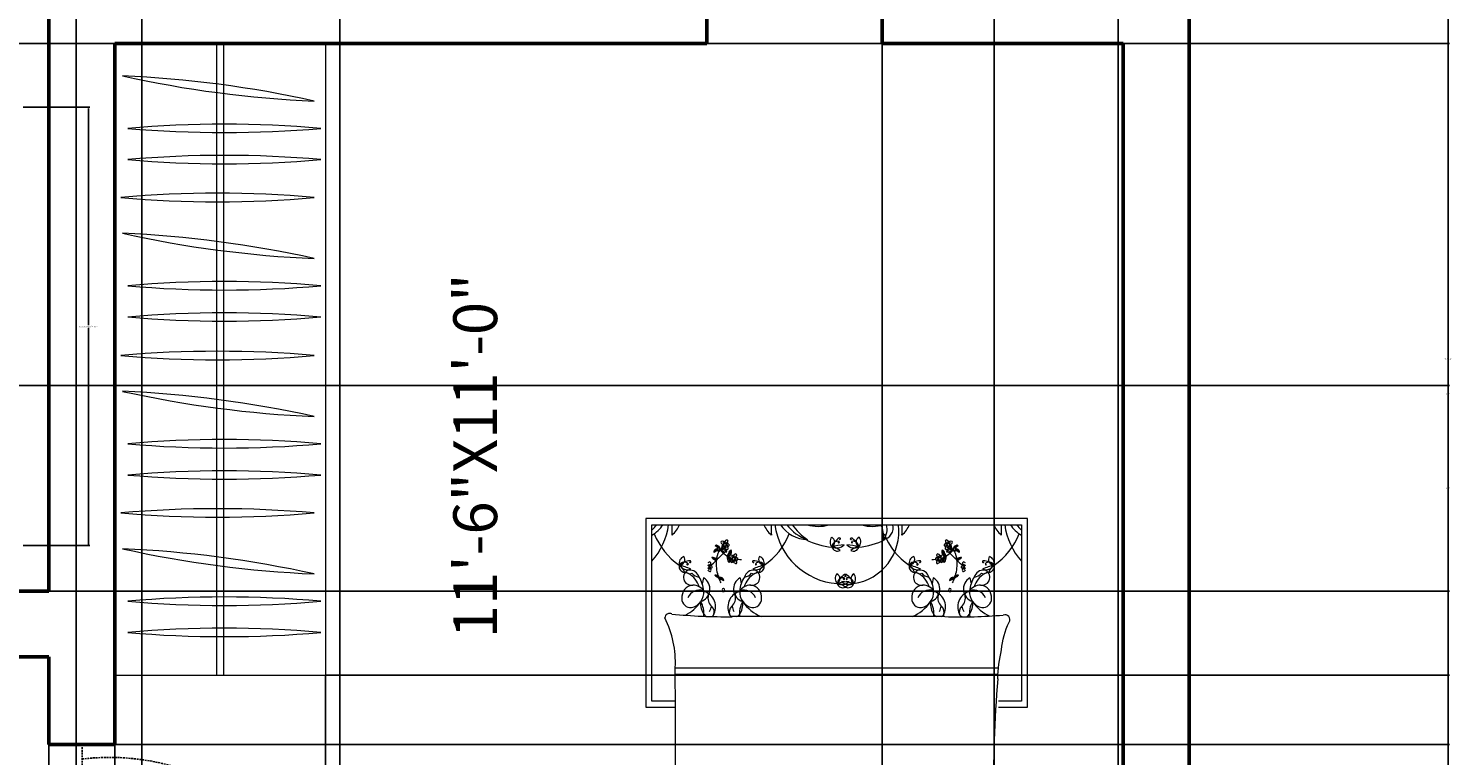
# Model space of a CAD drawing. Units: inches. Extents: x 3 to 576, y -689 to 51.
# Tile 20 of 21: x 381 to 576, y -148 to -48. Entities that reach past the tile are written whole.
import ezdxf

# ---------------------------------------------------------------- set-up
doc = ezdxf.new("R2010")
doc.units = ezdxf.units.IN
doc.header["$MEASUREMENT"] = 0
doc.linetypes.add('DASHED2', pattern=[0.375, 0.25, -0.125])
for name, color, linetype, lineweight in [('A-ANNO-DIMS', 2, 'Continuous', 18), ('A-AREA-IDEN', 7, 'Continuous', 18), ('A-DOOR', 4, 'DASHED2', 25), ('A-FURN', 8, 'Continuous', 18), ('A-WALL', 7, 'Continuous', 50)]:
    doc.layers.add(name, color=color, linetype=linetype, lineweight=lineweight)
doc.styles.get("Standard").update_dxf_attribs({"font": 'arial.ttf'})
doc.dimstyles.get("Standard").update_dxf_attribs({"dimtxt": 0.18, "dimasz": 0.18, "dimexe": 0.18, "dimexo": 0.0625, "dimgap": 0.09, "dimtad": 0, "dimtih": 1, "dimtoh": 1, "dimdec": 0, "dimzin": 0, "dimdsep": 46, "dimlunit": 3, "dimtxsty": 'Standard', "dimcen": 0.09, "dimadec": 0, "dimazin": 0, "dimtfac": 1, "dimtdec": 0, "dimtofl": 0, "dimtmove": 0, "dimatfit": 3, "dimfxl": 1, "dimtolj": 1, "dimtzin": 0, "dimarcsym": 0})

# ---------------------------------------------------------------- blocks, each defined once
blk = doc.blocks.new('DOOR-SWING-900')
for p, q in [((35.95, 36), (35.95, 34)), ((36, 2), (35.95, 34)), ((36, 2), (0, 2)), ((36, 0), (36, 2))]:
    blk.add_line(p, q)
blk.add_arc((32.22, 2), 32.22, 83.347, 180)
blk = doc.blocks.new('*D35')
at = {"layer": 'A-ANNO-DIMS', "color": 0, "lineweight": -2, "transparency": 16777216}
for p, q in [((380.75, -59.06), (389.87, -59.06)), ((389.69, -59.24), (389.69, -88.89)), ((389.69, -118.91), (389.69, -89.26)), ((380.75, -119.09), (389.87, -119.09))]:
    blk.add_line(p, q, dxfattribs=at)
at = {"layer": 'A-ANNO-DIMS', "color": 0, "transparency": 16777216}
for points in [[(389.66, -59.24), (389.72, -59.24), (389.69, -59.06)], [(389.66, -118.91), (389.72, -118.91), (389.69, -119.09)]]:
    blk.add_solid(points, dxfattribs=at)
at = {"layer": 'Defpoints', "color": 0, "transparency": 16777216}
for p in [(380.69, -59.06), (389.69, -59.06), (380.69, -119.09)]:
    blk.add_point(p, dxfattribs=at)
at = {"layer": 'A-ANNO-DIMS', "color": 0, "transparency": 16777216, "insert": (389.69, -89.08), "char_height": 0.18, "attachment_point": 5}
blk.add_mtext('\\A1;3-SEAT SOFA 5\'-0" TYP.', dxfattribs=at)
blk = doc.blocks.new('*D39')
at = {"layer": 'A-ANNO-DIMS', "color": 0, "lineweight": -2, "transparency": 16777216}
for p, q in [((540.36, 15.69), (575.92, 15.69)), ((575.74, 15.51), (575.74, -318.63)), ((575.74, -653.13), (575.74, -318.99)), ((540.36, -653.31), (575.92, -653.31))]:
    blk.add_line(p, q, dxfattribs=at)
at = {"layer": 'A-ANNO-DIMS', "color": 0, "transparency": 16777216}
for points in [[(575.71, 15.51), (575.77, 15.51), (575.74, 15.69)], [(575.71, -653.13), (575.77, -653.13), (575.74, -653.31)]]:
    blk.add_solid(points, dxfattribs=at)
at = {"layer": 'Defpoints', "color": 0, "transparency": 16777216}
for p in [(540.29, 15.69), (540.29, -653.31), (575.74, -653.31)]:
    blk.add_point(p, dxfattribs=at)
at = {"layer": 'A-ANNO-DIMS', "color": 0, "transparency": 16777216, "insert": (575.74, -318.81), "char_height": 0.18, "attachment_point": 5}
blk.add_mtext('\\A1;55\'-9"', dxfattribs=at)
blk = doc.blocks.new('*D64')
at = {"layer": 'A-ANNO-DIMS', "color": 0, "lineweight": -2, "transparency": 16777216}
for p, q in [((540.23, 15.69), (2.66, 15.69)), ((2.84, 15.51), (2.84, -17.13)), ((2.84, -50.13), (2.84, -17.49)), ((531.23, -50.31), (2.66, -50.31))]:
    blk.add_line(p, q, dxfattribs=at)
at = {"layer": 'A-ANNO-DIMS', "color": 0, "transparency": 16777216}
for points in [[(2.81, 15.51), (2.87, 15.51), (2.84, 15.69)], [(2.81, -50.13), (2.87, -50.13), (2.84, -50.31)]]:
    blk.add_solid(points, dxfattribs=at)
at = {"layer": 'Defpoints', "color": 0, "transparency": 16777216}
for p in [(540.29, 15.69), (2.84, -50.31), (531.29, -50.31)]:
    blk.add_point(p, dxfattribs=at)
at = {"layer": 'A-ANNO-DIMS', "color": 0, "transparency": 16777216, "insert": (2.84, -17.31), "char_height": 0.18, "attachment_point": 5}
blk.add_mtext('\\A1;5\'-6"', dxfattribs=at)
blk = doc.blocks.new('*D65')
at = {"layer": 'A-ANNO-DIMS', "color": 0, "lineweight": -2, "transparency": 16777216}
for p, q in [((531.23, -50.31), (2.66, -50.31)), ((2.84, -50.49), (2.84, -116.13)), ((2.84, -182.13), (2.84, -116.49)), ((531.23, -182.31), (2.66, -182.31))]:
    blk.add_line(p, q, dxfattribs=at)
at = {"layer": 'A-ANNO-DIMS', "color": 0, "transparency": 16777216}
for points in [[(2.81, -50.49), (2.87, -50.49), (2.84, -50.31)], [(2.81, -182.13), (2.87, -182.13), (2.84, -182.31)]]:
    blk.add_solid(points, dxfattribs=at)
at = {"layer": 'Defpoints', "color": 0, "transparency": 16777216}
for p in [(531.29, -50.31), (2.84, -182.31), (531.29, -182.31)]:
    blk.add_point(p, dxfattribs=at)
at = {"layer": 'A-ANNO-DIMS', "color": 0, "transparency": 16777216, "insert": (2.84, -116.31), "char_height": 0.18, "attachment_point": 5}
blk.add_mtext('\\A1;11\'-0"', dxfattribs=at)
blk = doc.blocks.new('*D87')
at = {"layer": 'A-ANNO-DIMS', "color": 0, "lineweight": -2, "transparency": 16777216}
for p, q in [((195.85, -97.15), (575.92, -97.15)), ((575.74, -97.33), (575.74, -111.05)), ((575.74, -125.13), (575.74, -111.41)), ((195.85, -125.31), (575.92, -125.31))]:
    blk.add_line(p, q, dxfattribs=at)
at = {"layer": 'A-ANNO-DIMS', "color": 0, "transparency": 16777216}
for points in [[(575.71, -97.33), (575.77, -97.33), (575.74, -97.15)], [(575.71, -125.13), (575.77, -125.13), (575.74, -125.31)]]:
    blk.add_solid(points, dxfattribs=at)
at = {"layer": 'Defpoints', "color": 0, "transparency": 16777216}
for p in [(195.78, -97.15), (575.74, -97.15), (195.78, -125.31)]:
    blk.add_point(p, dxfattribs=at)
at = {"layer": 'A-ANNO-DIMS', "color": 0, "transparency": 16777216, "insert": (575.74, -111.23), "char_height": 0.18, "attachment_point": 5}
blk.add_mtext('\\A1;2\'-4"', dxfattribs=at)
blk = doc.blocks.new('*D94')
at = {"layer": 'A-ANNO-DIMS', "color": 0, "lineweight": -2, "transparency": 16777216}
for p, q in [((393.29, -136.9), (393.29, -688.94)), ((422.14, -136.9), (422.14, -688.94)), ((393.47, -688.76), (407.39, -688.76)), ((421.96, -688.76), (408.05, -688.76))]:
    blk.add_line(p, q, dxfattribs=at)
at = {"layer": 'A-ANNO-DIMS', "color": 0, "transparency": 16777216}
for points in [[(393.47, -688.73), (393.47, -688.79), (393.29, -688.76)], [(421.96, -688.73), (421.96, -688.79), (422.14, -688.76)]]:
    blk.add_solid(points, dxfattribs=at)
at = {"layer": 'Defpoints', "color": 0, "transparency": 16777216}
for p in [(393.29, -136.84), (422.14, -136.84), (422.14, -688.76)]:
    blk.add_point(p, dxfattribs=at)
at = {"layer": 'A-ANNO-DIMS', "color": 0, "transparency": 16777216, "insert": (407.72, -688.76), "char_height": 0.18, "attachment_point": 5}
blk.add_mtext('\\A1;2\'-5"', dxfattribs=at)
blk = doc.blocks.new('*D95')
at = {"layer": 'A-ANNO-DIMS', "color": 0, "lineweight": -2, "transparency": 16777216}
for p, q in [((422.2, -50.31), (575.92, -50.31)), ((575.74, -50.49), (575.74, -93.39)), ((575.74, -136.66), (575.74, -93.76)), ((422.2, -136.84), (575.92, -136.84))]:
    blk.add_line(p, q, dxfattribs=at)
at = {"layer": 'A-ANNO-DIMS', "color": 0, "transparency": 16777216}
for points in [[(575.71, -50.49), (575.77, -50.49), (575.74, -50.31)], [(575.71, -136.66), (575.77, -136.66), (575.74, -136.84)]]:
    blk.add_solid(points, dxfattribs=at)
at = {"layer": 'Defpoints', "color": 0, "transparency": 16777216}
for p in [(422.14, -50.31), (422.14, -136.84), (575.74, -136.84)]:
    blk.add_point(p, dxfattribs=at)
at = {"layer": 'A-ANNO-DIMS', "color": 0, "transparency": 16777216, "insert": (575.74, -93.58), "char_height": 0.18, "attachment_point": 5}
blk.add_mtext('\\A1;7\'-2 1/2"', dxfattribs=at)
blk = doc.blocks.new('*D96')
at = {"layer": 'A-ANNO-DIMS', "color": 0, "lineweight": -2, "transparency": 16777216}
for p, q in [((397.02, -506.04), (397.02, 51.32)), ((397.2, 51.14), (410.22, 51.14)), ((423.91, 51.14), (410.89, 51.14)), ((424.09, -506.04), (424.09, 51.32))]:
    blk.add_line(p, q, dxfattribs=at)
at = {"layer": 'A-ANNO-DIMS', "color": 0, "transparency": 16777216}
for points in [[(397.2, 51.17), (397.2, 51.11), (397.02, 51.14)], [(423.91, 51.17), (423.91, 51.11), (424.09, 51.14)]]:
    blk.add_solid(points, dxfattribs=at)
at = {"layer": 'Defpoints', "color": 0, "transparency": 16777216}
for p in [(424.09, 51.14), (397.02, -506.1), (424.09, -506.1)]:
    blk.add_point(p, dxfattribs=at)
at = {"layer": 'A-ANNO-DIMS', "color": 0, "transparency": 16777216, "insert": (410.56, 51.14), "char_height": 0.18, "attachment_point": 5}
blk.add_mtext('\\A1;2\'-3"', dxfattribs=at)
blk = doc.blocks.new('*D103')
at = {"layer": 'A-ANNO-DIMS', "color": 0, "lineweight": -2, "transparency": 16777216}
for p, q in [((498.29, -50.37), (498.29, -688.94)), ((531.29, -50.37), (531.29, -688.94)), ((498.47, -688.76), (514.46, -688.76)), ((531.11, -688.76), (515.12, -688.76))]:
    blk.add_line(p, q, dxfattribs=at)
at = {"layer": 'A-ANNO-DIMS', "color": 0, "transparency": 16777216}
for points in [[(498.47, -688.73), (498.47, -688.79), (498.29, -688.76)], [(531.11, -688.73), (531.11, -688.79), (531.29, -688.76)]]:
    blk.add_solid(points, dxfattribs=at)
at = {"layer": 'Defpoints', "color": 0, "transparency": 16777216}
for p in [(498.29, -50.31), (531.29, -50.31), (531.29, -688.76)]:
    blk.add_point(p, dxfattribs=at)
at = {"layer": 'A-ANNO-DIMS', "color": 0, "transparency": 16777216, "insert": (514.79, -688.76), "char_height": 0.18, "attachment_point": 5}
blk.add_mtext('\\A1;2\'-9"', dxfattribs=at)
blk = doc.blocks.new('*D104')
at = {"layer": 'A-ANNO-DIMS', "color": 0, "lineweight": -2, "transparency": 16777216}
for p, q in [((393.36, -50.31), (575.92, -50.31)), ((575.74, -50.49), (575.74, -98.13)), ((575.74, -146.13), (575.74, -98.49)), ((393.36, -146.31), (575.92, -146.31))]:
    blk.add_line(p, q, dxfattribs=at)
at = {"layer": 'A-ANNO-DIMS', "color": 0, "transparency": 16777216}
for points in [[(575.71, -50.49), (575.77, -50.49), (575.74, -50.31)], [(575.71, -146.13), (575.77, -146.13), (575.74, -146.31)]]:
    blk.add_solid(points, dxfattribs=at)
at = {"layer": 'Defpoints', "color": 0, "transparency": 16777216}
for p in [(393.29, -50.31), (393.29, -146.31), (575.74, -146.31)]:
    blk.add_point(p, dxfattribs=at)
at = {"layer": 'A-ANNO-DIMS', "color": 0, "transparency": 16777216, "insert": (575.74, -98.31), "char_height": 0.18, "attachment_point": 5}
blk.add_mtext('\\A1;8\'-0"', dxfattribs=at)
blk = doc.blocks.new('*D116')
at = {"layer": 'A-ANNO-DIMS', "color": 0, "lineweight": -2, "transparency": 16777216}
for p, q in [((360.29, -134.37), (360.29, -688.94)), ((384.29, -134.37), (384.29, -688.94)), ((360.47, -688.76), (371.96, -688.76)), ((384.11, -688.76), (372.62, -688.76))]:
    blk.add_line(p, q, dxfattribs=at)
at = {"layer": 'A-ANNO-DIMS', "color": 0, "transparency": 16777216}
for points in [[(360.47, -688.73), (360.47, -688.79), (360.29, -688.76)], [(384.11, -688.73), (384.11, -688.79), (384.29, -688.76)]]:
    blk.add_solid(points, dxfattribs=at)
at = {"layer": 'Defpoints', "color": 0, "transparency": 16777216}
for p in [(360.29, -134.31), (384.29, -134.31), (384.29, -688.76)]:
    blk.add_point(p, dxfattribs=at)
at = {"layer": 'A-ANNO-DIMS', "color": 0, "transparency": 16777216, "insert": (372.29, -688.76), "char_height": 0.18, "attachment_point": 5}
blk.add_mtext('\\A1;2\'-0"', dxfattribs=at)
blk = doc.blocks.new('*D118')
at = {"layer": 'A-ANNO-DIMS', "color": 0, "lineweight": -2, "transparency": 16777216}
for p, q in [((352.02, -506.25), (352.02, 51.32)), ((352.2, 51.14), (369.69, 51.14)), ((387.84, 51.14), (370.35, 51.14)), ((388.02, -506.25), (388.02, 51.32))]:
    blk.add_line(p, q, dxfattribs=at)
at = {"layer": 'A-ANNO-DIMS', "color": 0, "transparency": 16777216}
for points in [[(352.2, 51.17), (352.2, 51.11), (352.02, 51.14)], [(387.84, 51.17), (387.84, 51.11), (388.02, 51.14)]]:
    blk.add_solid(points, dxfattribs=at)
at = {"layer": 'Defpoints', "color": 0, "transparency": 16777216}
for p in [(388.02, 51.14), (352.02, -506.31), (388.02, -506.31)]:
    blk.add_point(p, dxfattribs=at)
at = {"layer": 'A-ANNO-DIMS', "color": 0, "transparency": 16777216, "insert": (370.02, 51.14), "char_height": 0.18, "attachment_point": 5}
blk.add_mtext('\\A1;3\'-0"', dxfattribs=at)
blk = doc.blocks.new('*D124')
at = {"layer": 'A-ANNO-DIMS', "color": 0, "lineweight": -2, "transparency": 16777216}
for p, q in [((513.61, -235.44), (513.61, 51.32)), ((513.79, 51.14), (521.77, 51.14)), ((530.39, 51.14), (522.41, 51.14)), ((530.57, -227.22), (530.57, 51.32))]:
    blk.add_line(p, q, dxfattribs=at)
at = {"layer": 'A-ANNO-DIMS', "color": 0, "transparency": 16777216}
for points in [[(513.79, 51.17), (513.79, 51.11), (513.61, 51.14)], [(530.39, 51.17), (530.39, 51.11), (530.57, 51.14)]]:
    blk.add_solid(points, dxfattribs=at)
at = {"layer": 'Defpoints', "color": 0, "transparency": 16777216}
for p in [(530.57, 51.14), (530.57, -227.28), (513.61, -235.5)]:
    blk.add_point(p, dxfattribs=at)
at = {"layer": 'A-ANNO-DIMS', "color": 0, "transparency": 16777216, "insert": (522.09, 51.14), "char_height": 0.18, "attachment_point": 5}
blk.add_mtext('\\A1;1\'-5"', dxfattribs=at)

msp = doc.modelspace()

# ---------------------------------------------------------------- linework, layer by layer
at = {"layer": 'A-FURN'}
for p, q in [((393.29, -50.31), (393.29, -136.84)), ((393.29, -50.31), (422.14, -50.31)), ((407.24, -50.31), (407.24, -136.84)), ((408.2, -50.31), (408.2, -136.84)), ((422.14, -50.31), (422.14, -136.84)), ((465.95, -115.39), (465.95, -141.21)), ((518.2, -115.39), (465.95, -115.39)), ((466.78, -116.22), (517.37, -116.22)), ((466.78, -140.38), (466.78, -116.22)), ((517.37, -116.22), (517.37, -140.38)), ((518.2, -141.21), (518.2, -115.39)), ((473.84, -123.49), (473.69, -124.3)), ((478.85, -123.49), (479.01, -124.3)), ((505.3, -123.49), (505.14, -124.3)), ((510.31, -123.49), (510.47, -124.3)), ((506.87, -128.81), (477.78, -128.81)), ((514.22, -135.85), (470, -135.85)), ((393.29, -136.84), (422.14, -136.84)), ((514.15, -136.74), (470, -136.74)), ((465.95, -141.21), (470.01, -141.21)), ((470, -140.38), (466.78, -140.38)), ((517.37, -140.38), (514.21, -140.38)), ((514.23, -141.21), (518.2, -141.21))]:
    msp.add_line(p, q, dxfattribs=at)
for points in [[(470.03, -149.36, -0.001242), (470, -135.76, 0.127202), (468.56, -128.99)], [(514.13, -137.31, -0.056112), (514.65, -133.36, -0.095341), (515.66, -129.56)]]:
    msp.add_lwpolyline(points, format="xyb", dxfattribs=at)
for centre in [(476.79, -118.97), (477.98, -120.89), (506.17, -120.89), (507.36, -118.97)]:
    msp.add_circle(centre, 0.183, dxfattribs=at)
for centre, radius, start, end in [((427.2, 93.42), 151.77, 257.508, 267.5023), ((387.76, -206.38), 151.77, 77.508, 87.5023), ((408.29, -213.14), 151.77, 85.0028, 94.9972), ((408.29, 89.25), 151.77, 265.0028, 274.9972), ((408.29, -217.41), 151.77, 85.0028, 94.9972), ((408.29, 84.98), 151.77, 265.0028, 274.9972), ((407.36, -222.6), 151.77, 85.0028, 94.9972), ((407.36, 79.78), 151.77, 265.0028, 274.9972), ((427.2, 71.86), 151.77, 257.508, 267.5023), ((387.76, -227.94), 151.77, 77.508, 87.5023), ((408.29, -234.69), 151.77, 85.0028, 94.9972), ((408.29, 67.69), 151.77, 265.0028, 274.9972), ((408.29, -238.97), 151.77, 85.0028, 94.9972), ((408.29, 63.42), 151.77, 265.0028, 274.9972), ((407.36, -244.24), 151.77, 85.0028, 94.9972), ((407.36, 58.14), 151.77, 265.0028, 274.9972), ((387.76, -249.58), 151.77, 77.508, 87.5023), ((427.2, 50.22), 151.77, 257.508, 267.5023), ((408.29, -256.33), 151.77, 85.0028, 94.9972), ((408.29, 46.05), 151.77, 265.0028, 274.9972), ((408.29, -260.61), 151.77, 85.0028, 94.9972), ((408.29, 41.78), 151.77, 265.0028, 274.9972), ((407.36, -265.8), 151.77, 85.0028, 94.9972), ((407.36, 36.58), 151.77, 265.0028, 274.9972), ((462.87, -112.86), 5.68, 313.5186, 323.6964), ((464.51, -113.71), 4.56, 299.8884, 326.5383), ((459.81, -114.96), 9.36, 318.1144, 352.255), ((467.06, -114.76), 3.81, 311.0454, 337.4453), ((456.64, -116.81), 12.95, 356.3481, 2.5919), ((485.63, -114.76), 3.81, 202.5547, 228.9546), ((496.06, -116.81), 12.95, 177.4081, 183.6519), ((492.88, -114.96), 9.36, 187.745, 265.5377), ((488.19, -113.71), 4.56, 213.4617, 268.728), ((489.83, -112.86), 5.68, 216.3036, 252.1496), ((492.82, -111.26), 8.45, 215.947, 235.9877), ((489.55, -111.3), 5.15, 252.9798, 286.4569), ((491.59, -108.65), 7.61, 264.3643, 265.6213), ((495.6, -103.44), 13.6, 250.0972, 250.2783), ((493.35, -117.12), 7.24, 278.1803, 7.1364), ((496.99, -111.3), 5.15, 253.5431, 287.0202), ((494.95, -108.65), 7.61, 274.3787, 275.6357), ((490.94, -103.44), 13.6, 289.7217, 289.9028), ((494.29, -117.79), 4.19, 353.3805, 21.883), ((498.13, -116.62), 1.68, 280.9261, 13.6102), ((496.87, -116.85), 2.12, 318.0951, 17.1391), ((488.09, -116.81), 12.95, 356.3481, 2.5919), ((498.52, -114.76), 3.81, 311.0454, 337.4453), ((517.09, -114.76), 3.81, 202.5547, 228.9546), ((527.51, -116.81), 12.95, 177.4081, 183.6519), ((524.34, -114.96), 9.36, 187.745, 221.8856), ((519.64, -113.71), 4.56, 213.4617, 240.1116), ((521.28, -112.86), 5.68, 216.3036, 226.4814), ((475.83, -114.04), 9.36, 201.4092, 235.6135), ((476.41, -118.63), 0.181, 134.3732, 211.9501), ((476.74, -118.42), 0.575, 211.9501, 255.2442), ((476.42, -118.83), 0.36, 8.5614, 112.5914), ((476.52, -118.82), 0.121, 352.868, 97.094), ((477.04, -118.63), 0.301, 100.9597, 208.7804), ((477.36, -119.03), 0.554, 132.3896, 156.5724), ((476.78, -118.47), 0.424, 291.6382, 4.947), ((477.07, -118.45), 0.14, 4.947, 127.5263), ((476.87, -114.04), 9.36, 304.3865, 338.5908), ((492.17, -109.95), 9.36, 242.5854, 265.5377), ((492.21, -118.58), 1.04, 140.8855, 222.2127), ((491.03, -118.62), 0.782, 301.6373, 61.4609), ((493.68, -120.05), 2.37, 121.989, 161.0841), ((492.2, -119.25), 0.766, 76.148, 182.2415), ((492.36, -118.61), 0.101, 140.0755, 76.148), ((492.48, -118.14), 0.116, 288.4408, 121.989), ((492.5, -118.2), 0.0565, 171.9833, 288.4408), ((494.06, -118.14), 0.116, 58.011, 251.5592), ((494.04, -118.2), 0.0565, 251.5592, 8.0167), ((494.17, -118.64), 0.061, 103.9791, 39.8091), ((492.86, -120.05), 2.37, 18.9159, 58.011), ((494.34, -119.25), 0.766, 357.7585, 103.852), ((495.51, -118.62), 0.782, 118.5391, 238.3627), ((494.33, -118.58), 1.04, 317.7873, 39.1145), ((494.37, -109.95), 9.36, 274.4623, 297.4146), ((507.28, -114.04), 9.36, 201.4092, 235.6135), ((507.08, -118.45), 0.14, 52.4737, 175.053), ((507.37, -118.47), 0.424, 175.053, 248.3618), ((506.79, -119.03), 0.554, 23.4276, 47.6104), ((507.11, -118.63), 0.301, 331.2196, 79.0403), ((507.73, -118.83), 0.36, 67.4086, 171.4386), ((507.63, -118.82), 0.121, 82.906, 187.132), ((507.41, -118.42), 0.575, 284.7558, 328.0499), ((507.74, -118.63), 0.181, 328.0499, 45.6268), ((508.33, -114.04), 9.36, 304.3865, 338.5908), ((387.76, -271.14), 151.77, 77.508, 87.5023), ((427.2, 28.66), 151.77, 257.508, 267.5023), ((471.55, -121.54), 1.04, 110.9613, 192.2885), ((470.52, -120.98), 0.782, 271.7131, 31.5367), ((475.46, -119.9), 0.204, 123.0979, 213.1364), ((475.81, -120.2), 0.552, 92.3172, 160.5201), ((478.34, -124.39), 5.33, 121.1156, 124.8118), ((475.75, -119.99), 0.475, 82.6008, 147.1845), ((475.61, -119.24), 0.204, 55.6077, 145.6462), ((475.47, -119.67), 0.552, 21.7087, 93.0299), ((472.57, -123.61), 5.33, 53.6254, 57.3216), ((475.69, -120.01), 0.211, 45.7354, 121.1156), ((478.56, -121.35), 2.98, 150.7959, 175.244), ((482.85, -127.69), 9.79, 127.8256, 137.7588), ((475.64, -119.53), 0.475, 342.8042, 79.6943), ((475.6, -119.49), 0.211, 338.2452, 53.6254), ((475.95, -119.62), 0.159, 158.2452, 340.6395), ((475.95, -119.74), 0.159, 225.7354, 48.1297), ((478.94, -118.29), 3.18, 201.7087, 206.2181), ((476.41, -120.46), 0.832, 40.9365, 112.7695), ((476.14, -120.18), 0.49, 49.3812, 95.5456), ((478.56, -121.35), 2.98, 137.5083, 145.9967), ((476.49, -119.99), 0.506, 61.1838, 141.6792), ((478.87, -117.4), 3.57, 220.182, 239.456), ((476.59, -119.22), 0.249, 88.5719, 233.8954), ((476.56, -119.29), 0.179, 228.2946, 6.2474), ((476.84, -119.37), 0.589, 229.3812, 289.9959), ((476.39, -119.08), 0.251, 298.8493, 359.9355), ((476.45, -119.29), 0.287, 4.2123, 48.1587), ((477.04, -119.25), 0.304, 183.635, 258.4363), ((476.46, -120.08), 0.604, 15.6484, 62.2957), ((477, -119.14), 0.174, 178.1325, 268.8919), ((477.12, -119.1), 0.299, 42.3208, 130.2111), ((477.19, -118.79), 0.377, 226.3462, 279.6513), ((476.8, -119.49), 0.439, 7.4968, 71.2737), ((477.12, -118.4), 0.597, 254.2829, 276.9148), ((477.1, -119.47), 0.141, 215.0752, 14.7644), ((476.8, -119.69), 0.832, 287.889, 359.722), ((476.78, -120.08), 0.49, 305.1128, 351.2773), ((477.03, -120.98), 0.506, 3.8774, 87.1501), ((476.67, -120.78), 0.49, 352.0748, 38.2393), ((476.59, -121.16), 0.832, 343.6301, 55.4631), ((477.18, -119.99), 0.506, 271.4625, 339.4747), ((477.23, -119.01), 0.157, 279.6513, 42.3208), ((477.84, -120.24), 0.589, 110.6625, 171.2773), ((477.6, -120.55), 0.181, 134.3732, 211.9501), ((478.87, -117.4), 3.57, 246.1523, 246.9499), ((477.94, -120.34), 0.575, 211.9501, 255.2442), ((477.61, -120.75), 0.36, 8.5614, 112.5914), ((477.09, -119.95), 0.604, 338.3627, 25.0101), ((477.71, -120.74), 0.121, 352.868, 97.094), ((478.23, -120.56), 0.301, 100.9597, 208.7804), ((478.56, -120.96), 0.554, 132.3896, 156.5724), ((477.98, -120.4), 0.424, 291.6382, 4.947), ((478.26, -120.37), 0.14, 4.947, 127.5263), ((482.18, -120.98), 0.782, 148.4633, 268.2869), ((481.14, -121.54), 1.04, 347.7115, 69.0387), ((493.4, -125.53), 6.55, 92.7418, 107.407), ((492.05, -117.93), 1.48, 245.6899, 314.4589), ((491.4, -120.88), 1.6, 44.6273, 88.5415), ((492.18, -119.06), 0.776, 196.1963, 296.9726), ((493.14, -125.53), 6.55, 72.593, 87.2582), ((494.49, -117.93), 1.48, 225.5411, 294.3101), ((495.14, -120.88), 1.6, 91.4585, 135.3727), ((494.36, -119.06), 0.776, 243.0274, 343.8037), ((503.01, -121.54), 1.04, 110.9613, 192.2885), ((501.97, -120.98), 0.782, 271.7131, 31.5367), ((505.89, -120.37), 0.14, 52.4737, 175.053), ((506.17, -120.4), 0.424, 175.053, 248.3618), ((505.59, -120.96), 0.554, 23.4276, 47.6104), ((505.92, -120.56), 0.301, 331.2196, 79.0403), ((506.54, -120.75), 0.36, 67.4086, 171.4386), ((506.44, -120.74), 0.121, 82.906, 187.132), ((506.22, -120.34), 0.575, 284.7558, 328.0499), ((507.06, -119.95), 0.604, 154.9899, 201.6373), ((506.98, -119.99), 0.506, 200.5253, 268.5375), ((507.35, -119.69), 0.832, 180.278, 252.111), ((506.31, -120.24), 0.589, 8.7227, 69.3375), ((507.12, -120.98), 0.506, 92.8499, 176.1226), ((506.55, -120.55), 0.181, 328.0499, 45.6268), ((505.28, -117.4), 3.57, 293.0501, 293.8477), ((507.56, -121.16), 0.832, 124.5369, 196.3699), ((506.93, -119.01), 0.157, 137.6792, 260.3487), ((507.03, -119.1), 0.299, 49.7889, 137.6792), ((507.37, -120.08), 0.49, 188.7227, 234.8872), ((506.96, -118.79), 0.377, 260.3487, 313.6538), ((507.05, -119.47), 0.141, 165.2356, 324.9248), ((507.35, -119.49), 0.439, 108.7263, 172.5032), ((507.03, -118.4), 0.597, 263.0852, 285.7171), ((507.48, -120.78), 0.49, 141.7607, 187.9252), ((505.28, -117.4), 3.57, 300.544, 319.818), ((507.69, -120.08), 0.604, 117.7043, 164.3516), ((507.74, -120.46), 0.832, 67.2305, 139.0635), ((507.31, -119.37), 0.589, 250.0041, 310.6188), ((507.15, -119.14), 0.174, 271.1081, 1.8675), ((507.11, -119.25), 0.304, 281.5637, 356.365), ((501.3, -127.69), 9.79, 42.2412, 52.1744), ((507.7, -119.29), 0.287, 131.8413, 175.7877), ((507.59, -119.29), 0.179, 173.7526, 311.7054), ((507.66, -119.99), 0.506, 38.3208, 118.8162), ((507.76, -119.08), 0.251, 180.0645, 241.1507), ((507.56, -119.22), 0.249, 306.1046, 91.4281), ((508.01, -120.18), 0.49, 84.4544, 130.6188), ((505.59, -121.35), 2.98, 34.0033, 42.4917), ((508.51, -119.53), 0.475, 100.3057, 197.1958), ((508.2, -119.74), 0.159, 131.8703, 314.2646), ((508.2, -119.62), 0.159, 199.3605, 21.7548), ((505.21, -118.29), 3.18, 333.7819, 338.2913), ((508.68, -119.67), 0.552, 86.9701, 158.2913), ((505.59, -121.35), 2.98, 4.756, 29.2041), ((508.46, -120.01), 0.211, 58.8844, 134.2646), ((508.55, -119.49), 0.211, 126.3746, 201.7548), ((508.4, -119.99), 0.475, 32.8155, 97.3992), ((508.34, -120.2), 0.552, 19.4799, 87.6828), ((508.54, -119.24), 0.204, 34.3538, 124.3923), ((511.58, -123.61), 5.33, 122.6784, 126.3746), ((505.81, -124.39), 5.33, 55.1882, 58.8844), ((508.69, -119.9), 0.204, 326.8636, 56.9021), ((513.63, -120.98), 0.782, 148.4633, 268.2869), ((512.6, -121.54), 1.04, 347.7115, 69.0387), ((471.29, -121.95), 0.776, 166.272, 267.0484), ((472.1, -123.54), 2.37, 92.0648, 131.1598), ((471.22, -122.12), 0.766, 46.2238, 152.3173), ((469.12, -128.15), 6.55, 62.8176, 77.4827), ((471.74, -120.9), 1.48, 215.7657, 284.5347), ((469.71, -123.13), 1.6, 14.7031, 58.6173), ((472.2, -123.43), 1.08, 109.1312, 279.736), ((471.98, -122.27), 0.659, 216.7319, 296.0245), ((471.68, -121.64), 0.101, 110.2817, 46.2238), ((471.95, -123.76), 1.34, 15.6955, 94.031), ((472, -121.35), 0.0565, 142.0591, 258.5166), ((472.02, -121.29), 0.116, 258.5166, 92.0648), ((474.7, -121.64), 0.301, 100.9597, 142.2379), ((474.45, -121.98), 0.183, 273.2768, 86.7232), ((474.7, -122.26), 0.304, 217.3642, 258.4363), ((474.66, -122.15), 0.174, 178.1325, 268.8919), ((475.02, -122.04), 0.554, 132.3896, 156.5724), ((474.78, -122.11), 0.299, 42.3208, 130.2111), ((474.84, -121.8), 0.377, 226.3462, 279.6513), ((474.44, -121.48), 0.424, 291.6382, 4.947), ((474.45, -122.5), 0.439, 7.4968, 71.2737), ((474.77, -121.41), 0.597, 254.2829, 276.9148), ((474.72, -121.46), 0.14, 4.947, 127.5263), ((474.75, -122.48), 0.141, 215.0752, 14.7644), ((470.64, -116.45), 6.8, 307.9541, 316.8459), ((474.88, -122.02), 0.157, 279.6513, 42.3208), ((475.06, -122.74), 2.02, 82.8698, 91.6736), ((475.34, -120.56), 0.376, 205.5379, 258.6744), ((474.79, -121.84), 1.13, 59.344, 79.7412), ((474.55, -121.84), 1.15, 43.6929, 51.7899), ((475.26, -121.08), 0.344, 355.7131, 81.6568), ((475.07, -121.38), 0.601, 27.3659, 59.344), ((475.52, -120.98), 0.146, 202.5583, 304.2343), ((481.52, -121.5), 5.94, 176.1723, 196.4158), ((477.74, -120.93), 0.589, 172.0748, 232.6895), ((476.93, -121), 0.604, 318.342, 4.9894), ((477.78, -121.15), 0.249, 88.5719, 233.8954), ((477.76, -121.21), 0.179, 228.2946, 6.2474), ((477.59, -121), 0.251, 298.8493, 359.9355), ((477.65, -121.22), 0.287, 4.2123, 48.1587), ((478.24, -121.18), 0.304, 183.635, 258.4363), ((478.2, -121.07), 0.174, 178.1325, 268.8919), ((478.31, -121.03), 0.299, 42.3208, 130.2111), ((478.38, -120.72), 0.377, 226.3462, 279.6513), ((477.99, -121.41), 0.439, 7.4968, 71.2737), ((478.31, -120.32), 0.597, 254.2829, 276.9148), ((478.29, -121.39), 0.141, 215.0752, 14.7644), ((478.42, -120.93), 0.157, 279.6513, 42.3208), ((478.87, -117.4), 3.57, 265.2415, 272.8929), ((480.75, -123.76), 1.34, 85.969, 164.3045), ((480.49, -123.43), 1.08, 260.264, 70.8688), ((480.71, -122.27), 0.659, 243.9755, 323.2681), ((480.68, -121.29), 0.116, 87.9352, 281.4834), ((480.96, -120.9), 1.48, 255.4653, 324.2343), ((483.58, -128.15), 6.55, 102.5173, 117.1824), ((480.6, -123.54), 2.37, 48.8402, 87.9352), ((480.69, -121.35), 0.0565, 281.4834, 37.9409), ((481.48, -122.12), 0.766, 27.6827, 133.7762), ((481.03, -121.68), 0.061, 133.7729, 69.7333), ((481.4, -121.95), 0.776, 272.9516, 13.728), ((482.99, -123.13), 1.6, 121.3827, 165.2969), ((502.75, -121.95), 0.776, 166.272, 267.0484), ((503.55, -123.54), 2.37, 92.0648, 131.1598), ((502.67, -122.12), 0.766, 46.2238, 152.3173), ((501.16, -123.13), 1.6, 14.7031, 58.6173), ((503.19, -120.9), 1.48, 215.7657, 284.5347), ((500.58, -128.15), 6.55, 62.8176, 77.4827), ((503.66, -123.43), 1.08, 109.1312, 279.736), ((503.44, -122.27), 0.659, 216.7319, 296.0245), ((503.13, -121.64), 0.101, 110.2817, 46.2238), ((503.4, -123.76), 1.34, 15.6955, 94.031), ((503.46, -121.35), 0.0565, 142.0591, 258.5166), ((503.47, -121.29), 0.116, 258.5166, 92.0648), ((505.28, -117.4), 3.57, 267.1071, 274.7585), ((505.73, -120.93), 0.157, 137.6792, 260.3487), ((505.84, -121.03), 0.299, 49.7889, 137.6792), ((505.77, -120.72), 0.377, 260.3487, 313.6538), ((506.16, -121.41), 0.439, 108.7263, 172.5032), ((505.86, -121.39), 0.141, 165.2356, 324.9248), ((505.84, -120.32), 0.597, 263.0852, 285.7171), ((505.95, -121.07), 0.174, 271.1081, 1.8675), ((505.91, -121.18), 0.304, 281.5637, 356.365), ((506.5, -121.22), 0.287, 131.8413, 175.7877), ((506.4, -121.21), 0.179, 173.7526, 311.7054), ((506.56, -121), 0.251, 180.0645, 241.1507), ((506.37, -121.15), 0.249, 306.1046, 91.4281), ((507.22, -121), 0.604, 175.0106, 221.658), ((506.41, -120.93), 0.589, 307.3105, 7.9252), ((502.63, -121.5), 5.94, 343.5842, 3.8277), ((508.89, -121.08), 0.344, 98.3432, 184.2869), ((509.09, -121.38), 0.601, 120.656, 152.6341), ((508.63, -120.98), 0.146, 235.7657, 337.4417), ((513.52, -116.45), 6.8, 223.1541, 232.0459), ((509.6, -121.84), 1.15, 128.2101, 136.3071), ((509.36, -121.84), 1.13, 100.2588, 120.656), ((509.1, -122.74), 2.02, 88.3264, 97.1302), ((508.82, -120.56), 0.376, 281.3256, 334.4621), ((509.27, -122.02), 0.157, 137.6792, 260.3487), ((509.37, -122.11), 0.299, 49.7889, 137.6792), ((509.31, -121.8), 0.377, 260.3487, 313.6538), ((509.7, -122.5), 0.439, 108.7263, 172.5032), ((509.4, -122.48), 0.141, 165.2356, 324.9248), ((509.43, -121.46), 0.14, 52.4737, 175.053), ((509.71, -121.48), 0.424, 175.053, 248.3618), ((509.38, -121.41), 0.597, 263.0852, 285.7171), ((509.13, -122.04), 0.554, 23.4276, 47.6104), ((509.49, -122.15), 0.174, 271.1081, 1.8675), ((509.46, -121.64), 0.301, 37.7621, 79.0403), ((509.45, -122.26), 0.304, 281.5637, 322.6358), ((509.7, -121.98), 0.183, 93.2768, 266.7232), ((512.2, -123.76), 1.34, 85.969, 164.3045), ((511.95, -123.43), 1.08, 260.264, 70.8688), ((512.17, -122.27), 0.659, 243.9755, 323.2681), ((512.13, -121.29), 0.116, 87.9352, 281.4834), ((515.03, -128.15), 6.55, 102.5173, 117.1824), ((512.41, -120.9), 1.48, 255.4653, 324.2343), ((512.05, -123.54), 2.37, 48.8402, 87.9352), ((512.15, -121.35), 0.0565, 281.4834, 37.9409), ((512.93, -122.12), 0.766, 27.6827, 133.7762), ((512.48, -121.68), 0.061, 133.7729, 69.7333), ((514.44, -123.13), 1.6, 121.3827, 165.2969), ((512.86, -121.95), 0.776, 272.9516, 13.728), ((472.6, -126.19), 1.71, 97.1143, 185.0551), ((470.07, -125.8), 3.38, 18.2955, 58.7386), ((473.39, -121.97), 1.43, 218.4175, 263.8338), ((472.3, -126.57), 2.08, 35.9599, 87.6409), ((470.04, -125.53), 3.85, 3.4924, 33.7117), ((472.96, -125.03), 1.78, 286.8663, 60.0915), ((475.48, -125.16), 2.02, 82.8698, 91.6736), ((475.76, -122.97), 0.376, 205.5379, 258.6744), ((475.22, -124.25), 1.13, 59.344, 79.7412), ((474.98, -124.25), 1.15, 43.6929, 51.7899), ((475.68, -123.49), 0.344, 355.7131, 81.6568), ((475.49, -123.79), 0.601, 27.3659, 59.344), ((475.94, -123.4), 0.146, 202.5583, 304.2343), ((481.52, -121.5), 5.94, 200.1059, 206.9968), ((476.21, -123.81), 0.344, 36.5232, 122.4668), ((476.03, -124.12), 0.601, 58.836, 90.8141), ((476.17, -123.53), 0.146, 173.9457, 275.6216), ((475.88, -124.79), 1.15, 66.3901, 74.4871), ((476.63, -123.49), 0.376, 219.5056, 272.6421), ((475.76, -124.57), 1.13, 38.4388, 58.836), ((474.84, -124.77), 2.02, 26.5064, 35.3102), ((479.74, -125.03), 1.78, 119.9085, 253.1337), ((480.4, -126.57), 2.08, 92.3591, 144.0401), ((482.66, -125.53), 3.85, 146.2883, 176.5076), ((482.62, -125.8), 3.38, 121.2614, 161.7045), ((479.3, -121.97), 1.43, 276.1662, 321.5825), ((480.1, -126.19), 1.71, 354.9449, 82.8857), ((492.92, -123.6), 1.04, 140.8855, 222.2127), ((491.74, -123.63), 0.782, 301.6373, 61.4609), ((494.39, -125.06), 2.37, 121.989, 161.0841), ((492.92, -124.26), 0.766, 76.148, 182.2415), ((492.76, -122.95), 1.48, 245.6899, 314.4589), ((494.11, -130.54), 6.55, 92.7418, 107.407), ((492.9, -124.08), 0.776, 196.1963, 296.9726), ((492.11, -125.89), 1.6, 44.6273, 88.5415), ((493.78, -122.95), 1.48, 225.5411, 294.3101), ((492.43, -130.54), 6.55, 72.593, 87.2582), ((493.08, -123.62), 0.101, 140.0755, 76.148), ((493.2, -123.15), 0.116, 288.4408, 121.989), ((493.22, -123.21), 0.0565, 171.9833, 288.4408), ((493.34, -123.15), 0.116, 58.011, 251.5592), ((493.64, -124.08), 0.776, 243.0274, 343.8037), ((494.43, -125.89), 1.6, 91.4585, 135.3727), ((493.32, -123.21), 0.0565, 251.5592, 8.0167), ((493.45, -123.66), 0.061, 103.9791, 39.8091), ((492.15, -125.06), 2.37, 18.9159, 58.011), ((493.62, -124.26), 0.766, 357.7585, 103.852), ((494.8, -123.63), 0.782, 118.5391, 238.3627), ((493.62, -123.6), 1.04, 317.7873, 39.1145), ((504.05, -126.19), 1.71, 97.1143, 185.0551), ((501.53, -125.8), 3.38, 18.2955, 58.7386), ((504.85, -121.97), 1.43, 218.4175, 263.8338), ((503.76, -126.57), 2.08, 35.9599, 87.6409), ((501.49, -125.53), 3.85, 3.4924, 33.7117), ((504.41, -125.03), 1.78, 286.8663, 60.0915), ((508.39, -124.57), 1.13, 121.164, 141.5612), ((509.31, -124.77), 2.02, 144.6898, 153.4936), ((507.52, -123.49), 0.376, 267.3579, 320.4944), ((507.94, -123.81), 0.344, 57.5332, 143.4768), ((508.12, -124.12), 0.601, 89.1859, 121.164), ((508.27, -124.79), 1.15, 105.5129, 113.6099), ((502.63, -121.5), 5.94, 333.0032, 339.8941), ((507.98, -123.53), 0.146, 264.3784, 6.0543), ((508.47, -123.49), 0.344, 98.3432, 184.2869), ((508.66, -123.79), 0.601, 120.656, 152.6341), ((508.21, -123.4), 0.146, 235.7657, 337.4417), ((509.17, -124.25), 1.15, 128.2101, 136.3071), ((508.93, -124.25), 1.13, 100.2588, 120.656), ((508.67, -125.16), 2.02, 88.3264, 97.1302), ((508.39, -122.97), 0.376, 281.3256, 334.4621), ((511.2, -125.03), 1.78, 119.9085, 253.1337), ((511.85, -126.57), 2.08, 92.3591, 144.0401), ((514.11, -125.53), 3.85, 146.2883, 176.5076), ((514.08, -125.8), 3.38, 121.2614, 161.7045), ((510.76, -121.97), 1.43, 276.1662, 321.5825), ((511.55, -126.19), 1.71, 354.9449, 82.8857), ((408.29, -277.89), 151.77, 85.0028, 94.9972), ((472.1, -126.36), 1.21, 178.9462, 275.5144), ((473.27, -126.84), 1.66, 68.5779, 158.4181), ((471.73, -125.47), 2.16, 283.079, 4.7067), ((476.21, -126.99), 2.76, 143.6555, 147.2989), ((474.08, -125.78), 0.445, 344.8529, 102.6959), ((473.23, -127.51), 2.28, 330.8249, 70.7178), ((475.93, -126.28), 1.47, 164.8529, 228.4347), ((476.55, -125.11), 0.138, 79.5616, 257.2949), ((476.54, -125.19), 0.225, 259.5864, 79.5616), ((479.47, -127.51), 2.28, 109.2822, 209.1751), ((476.77, -126.28), 1.47, 311.5653, 15.1471), ((478.61, -125.78), 0.445, 77.3041, 195.1471), ((476.48, -126.99), 2.76, 32.7011, 36.3445), ((480.97, -125.47), 2.16, 175.2933, 256.921), ((479.43, -126.84), 1.66, 21.5819, 111.4221), ((480.59, -126.36), 1.21, 264.4856, 1.0538), ((503.56, -126.36), 1.21, 178.9462, 275.5144), ((504.73, -126.84), 1.66, 68.5779, 158.4181), ((503.19, -125.47), 2.16, 283.079, 4.7067), ((507.67, -126.99), 2.76, 143.6555, 147.2989), ((505.54, -125.78), 0.445, 344.8529, 102.6959), ((504.69, -127.51), 2.28, 330.8249, 70.7178), ((507.39, -126.28), 1.47, 164.8529, 228.4347), ((507.61, -125.19), 0.225, 100.4384, 280.4136), ((507.6, -125.11), 0.138, 282.7051, 100.4384), ((510.92, -127.51), 2.28, 109.2822, 209.1751), ((508.22, -126.28), 1.47, 311.5653, 15.1471), ((510.07, -125.78), 0.445, 77.3041, 195.1471), ((507.94, -126.99), 2.76, 32.7011, 36.3445), ((512.42, -125.47), 2.16, 175.2933, 256.921), ((510.88, -126.84), 1.66, 21.5819, 111.4221), ((512.05, -126.36), 1.21, 264.4856, 1.0538), ((408.29, 24.49), 151.77, 265.0028, 274.9972), ((469.22, -129.03), 0.661, 62.6588, 176.02), ((476.92, -54.21), 74.61, 264.3113, 270.6567), ((468.94, -123.76), 5.42, 296.7003, 326.3329), ((476.21, -126.99), 2.76, 175.2696, 214.215), ((470.93, -128.28), 2.97, 350.8446, 31.1782), ((472.89, -127.09), 2.06, 330.0851, 352.564), ((474.25, -128.19), 1.07, 336.1646, 48.4347), ((478.45, -128.19), 1.07, 131.5653, 203.8354), ((479.81, -127.09), 2.06, 187.436, 209.9149), ((476.48, -126.99), 2.76, 325.785, 4.7304), ((481.76, -128.28), 2.97, 148.8218, 190.2867), ((483.75, -123.76), 5.42, 213.6671, 248.5059), ((500.4, -123.76), 5.42, 291.4941, 326.3329), ((507.67, -126.99), 2.76, 175.2696, 214.215), ((502.39, -128.28), 2.97, 349.7133, 31.1782), ((504.34, -127.09), 2.06, 330.0851, 352.564), ((505.7, -128.19), 1.07, 336.1646, 48.4347), ((509.91, -128.19), 1.07, 131.5653, 203.8354), ((511.26, -127.09), 2.06, 187.436, 209.9149), ((507.94, -126.99), 2.76, 325.785, 4.7304), ((513.22, -128.28), 2.97, 148.8218, 190.751), ((515.21, -123.76), 5.42, 213.6671, 246.3547), ((408.29, -282.17), 151.77, 85.0028, 94.9972), ((474.61, -128.01), 0.863, 217.675, 239.9707), ((474.61, -128.01), 0.863, 296.442, 315.5483), ((478.09, -128.01), 0.863, 224.4517, 246.771), ((478.09, -128.01), 0.863, 293.2856, 322.325), ((506.06, -128.01), 0.863, 217.675, 246.7144), ((506.06, -128.01), 0.863, 293.2856, 315.5483), ((509.07, -59.1), 69.74, 268.1965, 274.7598), ((509.54, -128.01), 0.863, 224.4517, 253.3657), ((509.54, -128.01), 0.863, 287.4186, 322.325), ((515.12, -129.2), 0.653, 326.1736, 113.4781), ((408.29, 20.22), 151.77, 265.0028, 274.9972), ((681.5, -151.58), 167.98, 175.1265, 180.8855)]:
    msp.add_arc(centre, radius, start, end, dxfattribs=at)
at = {"layer": 'A-WALL'}
for p, q in [((540.29, 15.69), (540.29, -653.31)), ((474.29, 6.69), (474.29, -50.31)), ((384.29, -41.31), (384.29, -125.31)), ((498.29, -41.31), (498.29, -50.31)), ((393.29, -50.31), (465.29, -50.31)), ((393.29, -50.31), (393.29, -146.31)), ((465.29, -50.31), (474.29, -50.31)), ((498.29, -50.31), (531.29, -50.31)), ((531.29, -50.31), (531.29, -182.31)), ((360.29, -125.31), (384.29, -125.31)), ((360.29, -134.31), (384.29, -134.31)), ((384.29, -134.31), (384.29, -146.31)), ((393.29, -146.31), (384.29, -146.31))]:
    msp.add_line(p, q, dxfattribs=at)

# ---------------------------------------------------------------- block references
at = {"layer": 'A-DOOR', "extrusion": (0, 0, -1), "zscale": -1, "rotation": 359.9872034024854}
msp.add_blockref('DOOR-SWING-900', (-424.78, -182.3), dxfattribs=at)

# ---------------------------------------------------------------- texts
at = {"layer": 'A-AREA-IDEN', "insert": (439.62, -131.77), "char_height": 6, "attachment_point": 1, "rotation": 90}
msp.add_mtext('11\'-6"X11\'-0"', dxfattribs=at)

# ---------------------------------------------------------------- dimensions: what is measured, and where the dimension line sits
at = {"layer": 'A-ANNO-DIMS'}
for base, p1, p2, picture, middle in [((388.02, 51.14), (352.02, -506.31), (388.02, -506.31), '*D118', (370.02, 51.14)), ((424.09, 51.14), (397.02, -506.1), (424.09, -506.1), '*D96', (410.56, 51.14)), ((530.57, 51.14), (513.61, -235.5), (530.57, -227.28), '*D124', (522.09, 51.14)), ((531.29, -688.76), (498.29, -50.31), (531.29, -50.31), '*D103', (514.79, -688.76)), ((384.29, -688.76), (360.29, -134.31), (384.29, -134.31), '*D116', (372.29, -688.76)), ((422.1383, -688.7597), (393.294, -136.8425), (422.1383, -136.8425), '*D94', (407.7162, -688.7597))]:
    dim = msp.add_linear_dim(base=base, p1=p1, p2=p2, dimstyle='Standard', override={"dimdec": 1, "dimlfac": 1, "dimrnd": 0, "dimzin": 1, "dimdsep": 46, "dimlunit": 4, "dimfrac": 2}, dxfattribs=at)
    dim.commit()
    dim.dimension.update_dxf_attribs({"geometry": picture, "text_midpoint": middle})
for base, p1, p2, picture, middle in [((2.84, -50.31), (540.29, 15.69), (531.29, -50.31), '*D64', (2.84, -17.31)), ((575.74, -653.31), (540.29, 15.69), (540.29, -653.31), '*D39', (575.74, -318.81)), ((2.84, -182.31), (531.29, -50.31), (531.29, -182.31), '*D65', (2.84, -116.31)), ((575.74, -146.31), (393.29, -50.31), (393.29, -146.31), '*D104', (575.74, -98.31)), ((575.74, -136.84), (422.14, -50.31), (422.14, -136.84), '*D95', (575.74, -93.58)), ((575.74, -97.15), (195.78, -125.31), (195.78, -97.15), '*D87', (575.74, -111.23))]:
    dim = msp.add_linear_dim(base=base, p1=p1, p2=p2, angle=90, dimstyle='Standard', override={"dimdec": 1, "dimlfac": 1, "dimrnd": 0, "dimzin": 1, "dimdsep": 46, "dimlunit": 4, "dimfrac": 2}, dxfattribs=at)
    dim.commit()
    dim.dimension.update_dxf_attribs({"geometry": picture, "text_midpoint": middle})
dim = msp.add_linear_dim(base=(389.69, -59.06), p1=(380.69, -119.09), p2=(380.69, -59.06), angle=90, text='3-SEAT SOFA <> TYP.', dimstyle='Standard', override={"dimdec": 1, "dimlfac": 1, "dimrnd": 0, "dimzin": 1, "dimdsep": 46, "dimlunit": 4, "dimfrac": 2}, dxfattribs=at)
dim.commit()
dim.dimension.update_dxf_attribs({"geometry": '*D35', "text_midpoint": (389.69, -89.08)})

doc.saveas('drawing.dxf')
